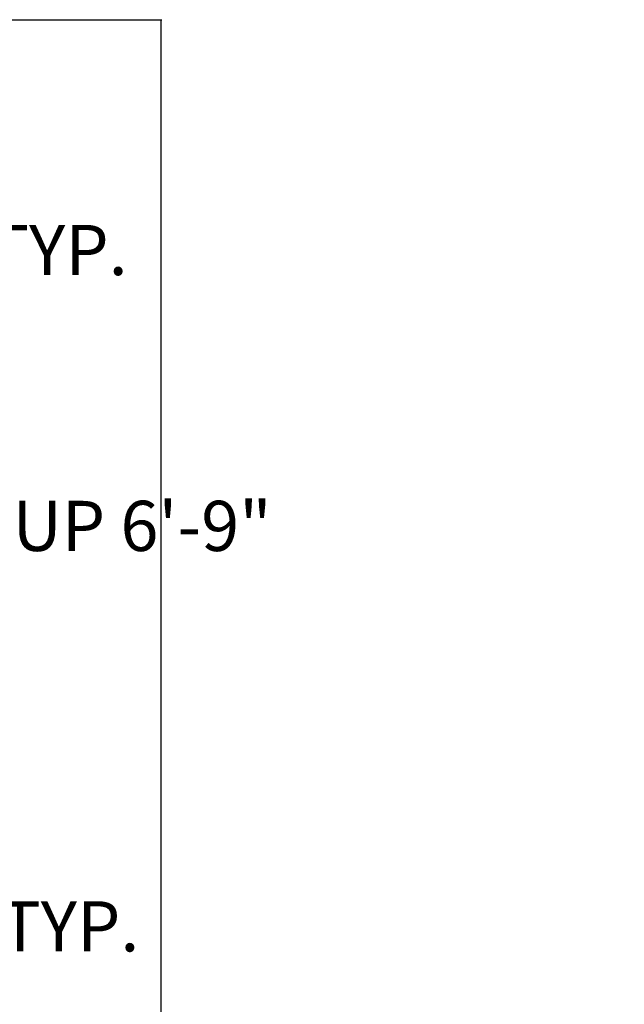
# Model space of a CAD drawing. Units: inches. Extents: x -4737294 to -4736756, y 1716389 to 1717040.
# Tile 25 of 25: x -4736853 to -4736756, y 1716845 to 1717002. Entities that reach past the tile are written whole.
import ezdxf

# ---------------------------------------------------------------- set-up
doc = ezdxf.new("R2010")
doc.units = ezdxf.units.IN
doc.header["$MEASUREMENT"] = 0
doc.layers.add('A-ANNO-DIMS', color=2, linetype='Continuous', lineweight=18)
doc.styles.get("Standard").update_dxf_attribs({"font": 'arial.ttf'})
doc.dimstyles.get("Standard").update_dxf_attribs({"dimtxt": 8, "dimasz": 0.18, "dimexe": 0.18, "dimexo": 0.0625, "dimgap": 0.09, "dimtad": 0, "dimtih": 1, "dimtoh": 1, "dimzin": 0, "dimdsep": 46, "dimlunit": 3, "dimtxsty": 'Standard', "dimcen": 0.09, "dimadec": 0, "dimazin": 0, "dimtfac": 1, "dimtofl": 0, "dimtmove": 0, "dimatfit": 3, "dimfxl": 1, "dimtolj": 1, "dimtzin": 0, "dimarcsym": 0})

# ---------------------------------------------------------------- blocks, each defined once
blk = doc.blocks.new('*D22')
at = {"layer": 'A-ANNO-DIMS', "color": 0, "lineweight": -2, "transparency": 16777216}
for p, q in [((-4736855.08, 1717002.06), (-4736830.06, 1717002.06)), ((-4736830.24, 1717001.88), (-4736830.24, 1716736.22)), ((-4736830.24, 1716462.24), (-4736830.24, 1716727.91)), ((-4736855.08, 1716462.06), (-4736830.06, 1716462.06))]:
    blk.add_line(p, q, dxfattribs=at)
at = {"layer": 'A-ANNO-DIMS', "color": 0, "transparency": 16777216}
for points in [[(-4736830.27, 1717001.88), (-4736830.21, 1717001.88), (-4736830.24, 1717002.06)], [(-4736830.27, 1716462.24), (-4736830.21, 1716462.24), (-4736830.24, 1716462.06)]]:
    blk.add_solid(points, dxfattribs=at)
at = {"layer": 'Defpoints', "color": 0, "transparency": 16777216}
for p in [(-4736855.14, 1717002.06), (-4736830.24, 1717002.06), (-4736855.14, 1716462.06)]:
    blk.add_point(p, dxfattribs=at)
at = {"layer": 'A-ANNO-DIMS', "color": 0, "transparency": 16777216, "insert": (-4736830.24, 1716732.06), "char_height": 8, "attachment_point": 5}
blk.add_mtext("\\A1;45'", dxfattribs=at)
blk = doc.blocks.new('*D27')
at = {"layer": 'A-ANNO-DIMS', "color": 0, "lineweight": -2, "transparency": 16777216}
for p, q in [((-4736969.31, 1716969), (-4736969.31, 1716965.16)), ((-4736944.45, 1716969), (-4736944.45, 1716965.16)), ((-4736969.13, 1716965.34), (-4736944.63, 1716965.34)), ((-4736944.45, 1716965.34), (-4736944.27, 1716965.34))]:
    blk.add_line(p, q, dxfattribs=at)
at = {"layer": 'A-ANNO-DIMS', "color": 0, "transparency": 16777216}
for points in [[(-4736969.13, 1716965.37), (-4736969.13, 1716965.31), (-4736969.31, 1716965.34)], [(-4736944.63, 1716965.37), (-4736944.63, 1716965.31), (-4736944.45, 1716965.34)]]:
    blk.add_solid(points, dxfattribs=at)
at = {"layer": 'Defpoints', "color": 0, "transparency": 16777216}
for p in [(-4736969.31, 1716969.06), (-4736944.45, 1716969.06), (-4736944.45, 1716965.34)]:
    blk.add_point(p, dxfattribs=at)
at = {"layer": 'A-ANNO-DIMS', "color": 0, "transparency": 16777216, "insert": (-4736888.21, 1716965.34), "char_height": 8, "attachment_point": 5}
blk.add_mtext('\\A1;ARMCHAIR 2\'-1" TYP.', dxfattribs=at)
blk = doc.blocks.new('*D35')
at = {"layer": 'A-ANNO-DIMS', "color": 0, "lineweight": -2, "transparency": 16777216}
for p, q in [((-4736868.27, 1716961.85), (-4736856.01, 1716961.83)), ((-4736856.19, 1716961.65), (-4736856.27, 1716925.58)), ((-4736856.37, 1716881.05), (-4736856.29, 1716917.12)), ((-4736868.45, 1716880.9), (-4736856.19, 1716880.87))]:
    blk.add_line(p, q, dxfattribs=at)
at = {"layer": 'A-ANNO-DIMS', "color": 0, "transparency": 16777216}
for points in [[(-4736856.22, 1716961.65), (-4736856.16, 1716961.65), (-4736856.19, 1716961.83)], [(-4736856.4, 1716881.05), (-4736856.34, 1716881.05), (-4736856.37, 1716880.87)]]:
    blk.add_solid(points, dxfattribs=at)
at = {"layer": 'Defpoints', "color": 0, "transparency": 16777216}
for p in [(-4736868.33, 1716961.85), (-4736868.51, 1716880.9), (-4736856.37, 1716880.87)]:
    blk.add_point(p, dxfattribs=at)
at = {"layer": 'A-ANNO-DIMS', "color": 0, "transparency": 16777216, "insert": (-4736856.28, 1716921.35), "char_height": 8, "attachment_point": 5}
blk.add_mtext('\\A1;BED GROUP 6\'-9"', dxfattribs=at)
blk = doc.blocks.new('*D47')
at = {"layer": 'A-ANNO-DIMS', "color": 0, "lineweight": -2, "transparency": 16777216}
for p, q in [((-4736950.1, 1716849.87), (-4736950.1, 1716837.75)), ((-4736870.07, 1716849.87), (-4736870.07, 1716837.75)), ((-4736949.92, 1716837.93), (-4736870.25, 1716837.93)), ((-4736870.07, 1716837.93), (-4736869.89, 1716837.93))]:
    blk.add_line(p, q, dxfattribs=at)
at = {"layer": 'A-ANNO-DIMS', "color": 0, "transparency": 16777216}
for points in [[(-4736949.92, 1716837.96), (-4736949.92, 1716837.9), (-4736950.1, 1716837.93)], [(-4736870.25, 1716837.96), (-4736870.25, 1716837.9), (-4736870.07, 1716837.93)]]:
    blk.add_solid(points, dxfattribs=at)
at = {"layer": 'Defpoints', "color": 0, "transparency": 16777216}
for p in [(-4736950.1, 1716849.93), (-4736870.07, 1716849.93), (-4736870.07, 1716837.93)]:
    blk.add_point(p, dxfattribs=at)
at = {"layer": 'A-ANNO-DIMS', "color": 0, "transparency": 16777216, "insert": (-4736810.8, 1716837.93), "char_height": 8, "attachment_point": 5}
blk.add_mtext('\\A1;WARDROBE 6\'-8" TYP.', dxfattribs=at)
blk = doc.blocks.new('*D48')
at = {"layer": 'A-ANNO-DIMS', "color": 0, "lineweight": -2, "transparency": 16777216}
for p, q in [((-4736870.01, 1716865.07), (-4736857.89, 1716865.07)), ((-4736858.07, 1716864.89), (-4736858.07, 1716861.68)), ((-4736858.07, 1716850.11), (-4736858.07, 1716853.32)), ((-4736870.01, 1716849.93), (-4736857.89, 1716849.93))]:
    blk.add_line(p, q, dxfattribs=at)
at = {"layer": 'A-ANNO-DIMS', "color": 0, "transparency": 16777216}
for points in [[(-4736858.1, 1716864.89), (-4736858.04, 1716864.89), (-4736858.07, 1716865.07)], [(-4736858.1, 1716850.11), (-4736858.04, 1716850.11), (-4736858.07, 1716849.93)]]:
    blk.add_solid(points, dxfattribs=at)
at = {"layer": 'Defpoints', "color": 0, "transparency": 16777216}
for p in [(-4736870.07, 1716865.07), (-4736858.07, 1716865.07), (-4736870.07, 1716849.93)]:
    blk.add_point(p, dxfattribs=at)
at = {"layer": 'A-ANNO-DIMS', "color": 0, "transparency": 16777216, "insert": (-4736858.07, 1716857.5), "char_height": 8, "attachment_point": 5}
blk.add_mtext('\\A1;1\'-3" TYP.', dxfattribs=at)

msp = doc.modelspace()

# ---------------------------------------------------------------- dimensions: what is measured, and where the dimension line sits
at = {"layer": 'A-ANNO-DIMS'}
dim = msp.add_linear_dim(base=(-4736830.238, 1717002.065), p1=(-4736855.144, 1716462.065), p2=(-4736855.144, 1717002.065), angle=90, dimstyle='Standard', override={"dimclrd": 0, "dimclre": 0, "dimclrt": 0}, dxfattribs=at)
dim.commit()
dim.dimension.update_dxf_attribs({"geometry": '*D22', "text_midpoint": (-4736830.238, 1716732.065)})
for base, p1, p2, text, picture, middle in [((-4736944.455, 1716965.337), (-4736969.306, 1716969.065), (-4736944.455, 1716969.065), 'ARMCHAIR <> TYP.', '*D27', (-4736888.215, 1716965.337)), ((-4736870.074, 1716837.93), (-4736950.098, 1716849.933), (-4736870.074, 1716849.933), 'WARDROBE <> TYP.', '*D47', (-4736810.797, 1716837.93))]:
    dim = msp.add_linear_dim(base=base, p1=p1, p2=p2, text=text, dimstyle='Standard', override={"dimdec": 1, "dimlfac": 1, "dimrnd": 0, "dimzin": 1, "dimdsep": 46, "dimlunit": 4, "dimfrac": 2}, dxfattribs=at)
    dim.commit()
    dim.dimension.update_dxf_attribs({"geometry": picture, "text_midpoint": middle})
for base, p1, p2, angle, text, picture, middle in [((-4736856.366, 1716880.874), (-4736868.335, 1716961.854), (-4736868.509, 1716880.9), 269.87691, 'BED GROUP <>', '*D35', (-4736856.279, 1716921.351)), ((-4736858.071, 1716865.067), (-4736870.074, 1716849.933), (-4736870.074, 1716865.067), 90, '<> TYP.', '*D48', (-4736858.071, 1716857.5))]:
    dim = msp.add_linear_dim(base=base, p1=p1, p2=p2, angle=angle, text=text, dimstyle='Standard', override={"dimdec": 1, "dimlfac": 1, "dimrnd": 0, "dimzin": 1, "dimdsep": 46, "dimlunit": 4, "dimfrac": 2}, dxfattribs=at)
    dim.commit()
    dim.dimension.update_dxf_attribs({"geometry": picture, "text_midpoint": middle})

doc.saveas('drawing.dxf')
